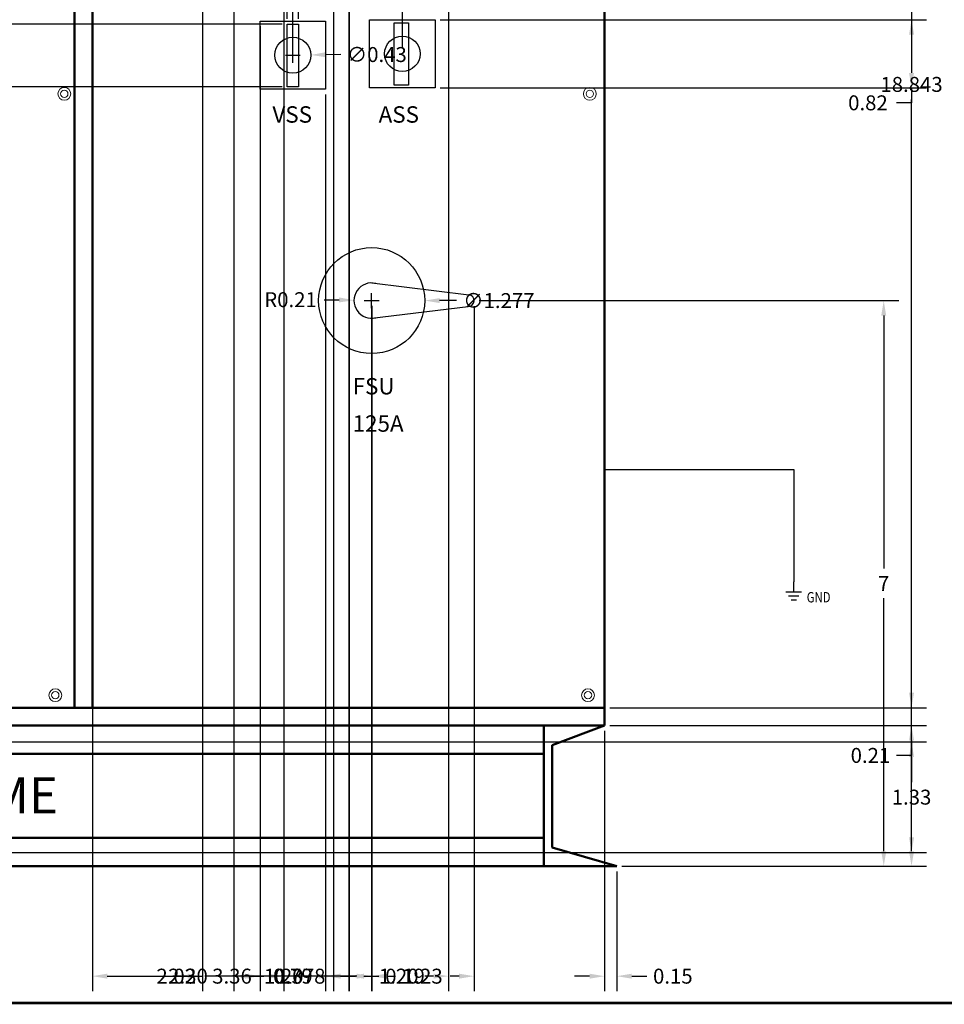
# Model space of a CAD drawing. Units: inches. Extents: x 0 to 33.5, y 0 to 22.4.
# Tile 4 of 6: x 16.8 to 27.9, y 0 to 11.9. Entities that reach past the tile are written whole.
import ezdxf
from ezdxf.enums import TextEntityAlignment as Align

# ---------------------------------------------------------------- set-up
doc = ezdxf.new("R2010")
doc.units = ezdxf.units.IN
doc.header["$MEASUREMENT"] = 0
for name, color, linetype, lineweight in [('E-ANNO-DIMS', 2, 'Continuous', 18), ('E-ANNO-TEXT', 7, 'Continuous', 18), ('E-ANNO-TTLB', 7, 'Continuous', 35), ('E-GRND-WIRE', 3, 'Continuous', 25), ('E-PANL-DEVC', 4, 'Continuous', 25), ('E-PANL-HDWR', 8, 'Continuous', 18), ('E-PANL-OUTL', 7, 'Continuous', 50), ('SYMS', 7, 'Continuous', 25)]:
    doc.layers.add(name, color=color, linetype=linetype, lineweight=lineweight)
doc.layers.add('TAGS', color=150, linetype='Continuous')
doc.layers.add('TITLE', color=7, linetype='Continuous')
doc.styles.add('ITALIC', font='ITALIC')
doc.styles.add('SIMPLEX', font='SIMPLEX')
doc.styles.add('WD', font='romans.shx')
doc.dimstyles.get("Standard").update_dxf_attribs({"dimtxt": 0.18, "dimasz": 0.18, "dimexe": 0.18, "dimexo": 0.0625, "dimgap": 0.09, "dimtad": 0, "dimtih": 1, "dimtoh": 1, "dimdec": 0, "dimzin": 0, "dimdsep": 46, "dimtxsty": 'Standard', "dimcen": 0.09, "dimadec": 0, "dimazin": 0, "dimtfac": 1, "dimtdec": 0, "dimtofl": 0, "dimtmove": 0, "dimatfit": 3, "dimfxl": 1, "dimtolj": 1, "dimtzin": 0, "dimarcsym": 0})

# ---------------------------------------------------------------- blocks, each defined once
blk = doc.blocks.new('NO_NUM_acade_title')
at = {"layer": 'TITLE', "const_width": 0.0312}
blk.add_lwpolyline([(30.594, 0.281), (30.594, 22.177), (30.344, 22.427), (0.281, 22.427), (0.031, 22.177), (0.031, 0.281), (0.281, 0.031), (30.344, 0.031)], close=True, dxfattribs=at)
at = {"layer": 'TITLE', "style": 'ITALIC'}
for tag, height, p in [('TITLE#1', 0.125, (32.156, 3.406)), ('TITLE#2', 0.125, (32.156, 3.204)), ('TITLE#3', 0.125, (32.156, 3.001)), ('TITLE#4', 0.125, (32.156, 2.799)), ('DWG#', 0.2, (32.156, 0.826))]:
    blk.add_attdef(tag, text='', height=height, dxfattribs=at).set_placement(p, align=Align.CENTER)
at = {"layer": 'TITLE', "style": 'SIMPLEX'}
blk.add_attdef('CAD#', (30.826, 1.958), '', height=0.0938, rotation=90, dxfattribs=at)
at = {"layer": 'TITLE'}
for tag, p, height, style in [('JOB#', (31.464, 1.644), 0.0938, 'SIMPLEX'), ('SCALE', (31.353, 1.344), 0.0938, 'SIMPLEX'), ('DATE', (32.408, 1.344), 0.0938, 'SIMPLEX'), ('SHTS', (32.532, 0.25), 0.2, 'ITALIC')]:
    blk.add_attdef(tag, p, '', height=height, dxfattribs=dict(at, style=style))
at = {"layer": 'TITLE', "style": 'ITALIC'}
blk.add_attdef('SH#', text='', height=0.2, dxfattribs=at).set_placement((31.881, 0.25), align=Align.RIGHT)
at = {"layer": 'TITLE', "flags": 9}
blk.add_attdef('WD_TB', (31.219, 0.031), '', height=0.125, dxfattribs=at)
blk = doc.blocks.new('VGND2')
for p, q in [((0, -0.125), (0, 0)), ((0.09375, -0.125), (-0.09375, -0.125)), ((-0.0625, -0.171875), (0.0625, -0.171875)), ((-0.03125, -0.21875), (0.03125, -0.21875))]:
    blk.add_line(p, q)
at = {"style": 'WD', "width": 0.8}
for tag, p in [('INST', (0.15625, 0.125)), ('LOC', (0.15625, -0.03125)), ('TAG1', (0.15625, -0.1875)), ('DESC1', (0.15625, -0.34375)), ('DESC2', (0.15625, -0.5))]:
    blk.add_attdef(tag, text='', height=0.125, dxfattribs=at).set_placement(p, align=Align.MIDDLE_LEFT)
at = {"style": 'WD', "flags": 1}
for tag in ['ASSYCODE', 'X2TERM01', 'CAT', 'MFG', 'FAMILY']:
    blk.add_attdef(tag, (0, 0), '', height=0.01, dxfattribs=at)
blk = doc.blocks.new('*D22')
at = {"layer": 'Defpoints', "color": 0, "transparency": 16777216}
for p in [(22.223, 8.496), (27.157, 8.496), (23.942, 1.68)]:
    blk.add_point(p, dxfattribs=at)
at = {"layer": 'E-ANNO-DIMS', "color": 0, "lineweight": -2, "transparency": 16777216}
for p, q in [((22.285, 8.496), (27.337, 8.496)), ((27.157, 8.316), (27.157, 5.268)), ((27.157, 1.86), (27.157, 4.908)), ((24.004, 1.68), (27.337, 1.68))]:
    blk.add_line(p, q, dxfattribs=at)
at = {"layer": 'E-ANNO-DIMS', "color": 0, "transparency": 16777216}
for points in [[(27.127, 8.316), (27.187, 8.316), (27.157, 8.496)], [(27.127, 1.86), (27.187, 1.86), (27.157, 1.68)]]:
    blk.add_solid(points, dxfattribs=at)
at = {"layer": 'E-ANNO-DIMS', "color": 0, "transparency": 16777216, "insert": (27.157, 5.088), "char_height": 0.18, "attachment_point": 5}
blk.add_mtext('\\A1;7', dxfattribs=at)
blk = doc.blocks.new('SCREW-PANEL')
for radius in [0.0768, 0.0442]:
    blk.add_circle((0.077, 0.077), radius)
blk = doc.blocks.new('*D31')
at = {"layer": 'Defpoints', "color": 0, "transparency": 16777216}
for p in [(14.887335, 20.522539), (27.49197, 20.522539), (23.941819, 1.679641)]:
    blk.add_point(p, dxfattribs=at)
at = {"layer": 'E-ANNO-DIMS', "color": 0, "lineweight": -2, "transparency": 16777216}
for p, q in [((14.949835, 20.522539), (27.67197, 20.522539)), ((27.49197, 20.342539), (27.49197, 11.28109)), ((27.49197, 1.859641), (27.49197, 10.92109)), ((24.004319, 1.679641), (27.67197, 1.679641))]:
    blk.add_line(p, q, dxfattribs=at)
at = {"layer": 'E-ANNO-DIMS', "color": 0, "transparency": 16777216}
for points in [[(27.46197, 20.342539), (27.52197, 20.342539), (27.49197, 20.522539)], [(27.46197, 1.859641), (27.52197, 1.859641), (27.49197, 1.679641)]]:
    blk.add_solid(points, dxfattribs=at)
at = {"layer": 'E-ANNO-DIMS', "color": 0, "transparency": 16777216, "insert": (27.49197, 11.10109), "char_height": 0.18, "attachment_point": 5}
blk.add_mtext('\\A1;18.843', dxfattribs=at)
blk = doc.blocks.new('*D32')
at = {"layer": 'Defpoints', "color": 0, "transparency": 16777216}
for p in [(23.793662, 3.589871), (23.793662, 3.375), (27.49197, 3.375)]:
    blk.add_point(p, dxfattribs=at)
at = {"layer": 'E-ANNO-DIMS', "color": 0, "lineweight": -2, "transparency": 16777216}
for p, q in [((27.49197, 3.769871), (27.49197, 3.949871)), ((23.856162, 3.589871), (27.67197, 3.589871)), ((23.856162, 3.375), (27.67197, 3.375)), ((27.49197, 3.195), (27.49197, 3.015)), ((27.49197, 3.015), (27.31197, 3.015))]:
    blk.add_line(p, q, dxfattribs=at)
at = {"layer": 'E-ANNO-DIMS', "color": 0, "transparency": 16777216}
for points in [[(27.46197, 3.769871), (27.52197, 3.769871), (27.49197, 3.589871)], [(27.46197, 3.195), (27.52197, 3.195), (27.49197, 3.375)]]:
    blk.add_solid(points, dxfattribs=at)
at = {"layer": 'E-ANNO-DIMS', "color": 0, "transparency": 16777216, "insert": (26.99697, 3.015), "char_height": 0.18, "attachment_point": 5}
blk.add_mtext('\\A1;0.21', dxfattribs=at)
blk = doc.blocks.new('*D33')
at = {"layer": 'Defpoints', "color": 0, "transparency": 16777216}
for p in [(23.061914, 3.375), (1.272879, 3.034671), (23.061914, 3.034671)]:
    blk.add_point(p, dxfattribs=at)
at = {"layer": 'E-ANNO-DIMS', "color": 0, "lineweight": -2, "transparency": 16777216}
for p, q in [((1.272879, 3.555), (1.272879, 3.735)), ((22.999414, 3.375), (1.092879, 3.375)), ((22.999414, 3.034671), (1.092879, 3.034671)), ((1.272879, 2.854671), (1.272879, 2.674671)), ((1.272879, 2.674671), (1.092879, 2.674671))]:
    blk.add_line(p, q, dxfattribs=at)
at = {"layer": 'E-ANNO-DIMS', "color": 0, "transparency": 16777216}
for points in [[(1.242879, 3.555), (1.302879, 3.555), (1.272879, 3.375)], [(1.242879, 2.854671), (1.302879, 2.854671), (1.272879, 3.034671)]]:
    blk.add_solid(points, dxfattribs=at)
at = {"layer": 'E-ANNO-DIMS', "color": 0, "transparency": 16777216, "insert": (0.747879, 2.674671), "char_height": 0.18, "attachment_point": 5}
blk.add_mtext('\\A1;0.34', dxfattribs=at)
blk = doc.blocks.new('*D34')
at = {"layer": 'Defpoints', "color": 0, "transparency": 16777216}
for p in [(23.061914, 2.019969), (1.272879, 1.679641), (23.061914, 1.679641)]:
    blk.add_point(p, dxfattribs=at)
at = {"layer": 'E-ANNO-DIMS', "color": 0, "lineweight": -2, "transparency": 16777216}
for p, q in [((1.272879, 2.199969), (1.272879, 2.379969)), ((22.999414, 2.019969), (1.092879, 2.019969)), ((22.999414, 1.679641), (1.092879, 1.679641)), ((1.272879, 1.499641), (1.272879, 1.319641)), ((1.272879, 1.319641), (1.092879, 1.319641))]:
    blk.add_line(p, q, dxfattribs=at)
at = {"layer": 'E-ANNO-DIMS', "color": 0, "transparency": 16777216}
for points in [[(1.242879, 2.199969), (1.302879, 2.199969), (1.272879, 2.019969)], [(1.242879, 1.499641), (1.302879, 1.499641), (1.272879, 1.679641)]]:
    blk.add_solid(points, dxfattribs=at)
at = {"layer": 'E-ANNO-DIMS', "color": 0, "transparency": 16777216, "insert": (0.747879, 1.319641), "char_height": 0.18, "attachment_point": 5}
blk.add_mtext('\\A1;0.34', dxfattribs=at)
blk = doc.blocks.new('*D37')
at = {"layer": 'Defpoints', "color": 0, "transparency": 16777216}
for p in [(5.494, 3.177), (5.494, 1.847), (27.492, 1.847)]:
    blk.add_point(p, dxfattribs=at)
at = {"layer": 'E-ANNO-DIMS', "color": 0, "lineweight": -2, "transparency": 16777216}
for p, q in [((5.557, 3.177), (27.672, 3.177)), ((27.492, 2.997), (27.492, 2.692)), ((27.492, 2.027), (27.492, 2.332)), ((5.557, 1.847), (27.672, 1.847))]:
    blk.add_line(p, q, dxfattribs=at)
at = {"layer": 'E-ANNO-DIMS', "color": 0, "transparency": 16777216}
for points in [[(27.462, 2.997), (27.522, 2.997), (27.492, 3.177)], [(27.462, 2.027), (27.522, 2.027), (27.492, 1.847)]]:
    blk.add_solid(points, dxfattribs=at)
at = {"layer": 'E-ANNO-DIMS', "color": 0, "transparency": 16777216, "insert": (27.492, 2.512), "char_height": 0.18, "attachment_point": 5}
blk.add_mtext('\\A1;1.33', dxfattribs=at)
blk = doc.blocks.new('*D38')
at = {"layer": 'Defpoints', "color": 0, "transparency": 16777216}
for p in [(23.793662, 3.375), (23.941819, 1.679641), (23.941819, 0.354641)]:
    blk.add_point(p, dxfattribs=at)
at = {"layer": 'E-ANNO-DIMS', "color": 0, "lineweight": -2, "transparency": 16777216}
for p, q in [((23.793662, 3.3125), (23.793662, 0.174641)), ((23.941819, 1.617141), (23.941819, 0.174641)), ((23.613662, 0.354641), (23.433662, 0.354641)), ((24.121819, 0.354641), (24.301819, 0.354641))]:
    blk.add_line(p, q, dxfattribs=at)
at = {"layer": 'E-ANNO-DIMS', "color": 0, "transparency": 16777216}
for points in [[(23.613662, 0.384641), (23.613662, 0.324641), (23.793662, 0.354641)], [(24.121819, 0.384641), (24.121819, 0.324641), (23.941819, 0.354641)]]:
    blk.add_solid(points, dxfattribs=at)
at = {"layer": 'E-ANNO-DIMS', "color": 0, "transparency": 16777216, "insert": (24.616819, 0.354641), "char_height": 0.18, "attachment_point": 5}
blk.add_mtext('\\A1;0.15', dxfattribs=at)
blk = doc.blocks.new('*D68')
at = {"layer": 'Defpoints', "color": 0, "transparency": 16777216}
for p in [(19.330943, 14.658017), (18.952991, 14.454443), (19.330943, 0.354641)]:
    blk.add_point(p, dxfattribs=at)
at = {"layer": 'E-ANNO-DIMS', "color": 0, "lineweight": -2, "transparency": 16777216}
for p, q in [((19.330943, 14.595517), (19.330943, 0.174641)), ((18.952991, 14.391943), (18.952991, 0.174641)), ((18.772991, 0.354641), (18.592991, 0.354641)), ((19.510943, 0.354641), (19.690943, 0.354641))]:
    blk.add_line(p, q, dxfattribs=at)
at = {"layer": 'E-ANNO-DIMS', "color": 0, "transparency": 16777216}
for points in [[(18.772991, 0.384641), (18.772991, 0.324641), (18.952991, 0.354641)], [(19.510943, 0.384641), (19.510943, 0.324641), (19.330943, 0.354641)]]:
    blk.add_solid(points, dxfattribs=at)
at = {"layer": 'E-ANNO-DIMS', "color": 0, "transparency": 16777216, "insert": (20.125943, 0.354641), "char_height": 0.18, "attachment_point": 5}
blk.add_mtext('\\A1;0.378', dxfattribs=at)
blk = doc.blocks.new('*D69')
at = {"layer": 'Defpoints', "color": 0, "transparency": 16777216}
for p in [(19.330943, 14.658017), (20.529167, 14.658017), (20.529167, 0.354641)]:
    blk.add_point(p, dxfattribs=at)
at = {"layer": 'E-ANNO-DIMS', "color": 0, "lineweight": -2, "transparency": 16777216}
for p, q in [((19.330943, 14.595517), (19.330943, 0.174641)), ((20.529167, 14.595517), (20.529167, 0.174641)), ((19.510943, 0.354641), (19.615055, 0.354641)), ((20.349167, 0.354641), (20.245055, 0.354641))]:
    blk.add_line(p, q, dxfattribs=at)
at = {"layer": 'E-ANNO-DIMS', "color": 0, "transparency": 16777216}
for points in [[(19.510943, 0.384641), (19.510943, 0.324641), (19.330943, 0.354641)], [(20.349167, 0.384641), (20.349167, 0.324641), (20.529167, 0.354641)]]:
    blk.add_solid(points, dxfattribs=at)
at = {"layer": 'E-ANNO-DIMS', "color": 0, "transparency": 16777216, "insert": (19.930055, 0.354641), "char_height": 0.18, "attachment_point": 5}
blk.add_mtext('\\A1;1.20', dxfattribs=at)
blk = doc.blocks.new('*D70')
at = {"layer": 'Defpoints', "color": 0, "transparency": 16777216}
for p in [(20.529167, 14.658017), (20.716317, 14.66483), (20.716317, 0.354641)]:
    blk.add_point(p, dxfattribs=at)
at = {"layer": 'E-ANNO-DIMS', "color": 0, "lineweight": -2, "transparency": 16777216}
for p, q in [((20.529167, 14.595517), (20.529167, 0.174641)), ((20.716317, 14.60233), (20.716317, 0.174641)), ((20.349167, 0.354641), (20.169167, 0.354641)), ((20.896317, 0.354641), (21.076317, 0.354641))]:
    blk.add_line(p, q, dxfattribs=at)
at = {"layer": 'E-ANNO-DIMS', "color": 0, "transparency": 16777216}
for points in [[(20.349167, 0.384641), (20.349167, 0.324641), (20.529167, 0.354641)], [(20.896317, 0.384641), (20.896317, 0.324641), (20.716317, 0.354641)]]:
    blk.add_solid(points, dxfattribs=at)
at = {"layer": 'E-ANNO-DIMS', "color": 0, "transparency": 16777216, "insert": (21.391317, 0.354641), "char_height": 0.18, "attachment_point": 5}
blk.add_mtext('\\A1;0.19', dxfattribs=at)
blk = doc.blocks.new('*D71')
at = {"layer": 'Defpoints', "color": 0, "transparency": 16777216}
for p in [(20.716, 14.665), (21.915, 14.665), (21.915, 0.355)]:
    blk.add_point(p, dxfattribs=at)
at = {"layer": 'E-ANNO-DIMS', "color": 0, "lineweight": -2, "transparency": 16777216}
for p, q in [((20.716, 14.602), (20.716, 0.175)), ((21.915, 14.602), (21.915, 0.175)), ((20.896, 0.355), (21, 0.355)), ((21.735, 0.355), (21.63, 0.355))]:
    blk.add_line(p, q, dxfattribs=at)
at = {"layer": 'E-ANNO-DIMS', "color": 0, "transparency": 16777216}
for points in [[(20.896, 0.385), (20.896, 0.325), (20.716, 0.355)], [(21.735, 0.385), (21.735, 0.325), (21.915, 0.355)]]:
    blk.add_solid(points, dxfattribs=at)
at = {"layer": 'E-ANNO-DIMS', "color": 0, "transparency": 16777216, "insert": (21.315, 0.355), "char_height": 0.18, "attachment_point": 5}
blk.add_mtext('\\A1;1.20', dxfattribs=at)
blk = doc.blocks.new('*D74')
at = {"layer": 'Defpoints', "color": 0, "transparency": 16777216}
for p in [(17.625, 18.375), (19.93, 13.017), (19.93, 0.355)]:
    blk.add_point(p, dxfattribs=at)
at = {"layer": 'E-ANNO-DIMS', "color": 0, "lineweight": -2, "transparency": 16777216}
for p, q in [((17.625, 18.312), (17.625, 0.175)), ((19.93, 12.954), (19.93, 0.175)), ((17.805, 0.355), (18.432, 0.355)), ((19.75, 0.355), (19.122, 0.355))]:
    blk.add_line(p, q, dxfattribs=at)
at = {"layer": 'E-ANNO-DIMS', "color": 0, "transparency": 16777216}
for points in [[(17.805, 0.385), (17.805, 0.325), (17.625, 0.355)], [(19.75, 0.385), (19.75, 0.325), (19.93, 0.355)]]:
    blk.add_solid(points, dxfattribs=at)
at = {"layer": 'E-ANNO-DIMS', "color": 0, "transparency": 16777216, "insert": (18.777, 0.355), "char_height": 0.18, "attachment_point": 5}
blk.add_mtext('\\A1;2.30', dxfattribs=at)
blk = doc.blocks.new('*D80')
at = {"layer": 'Defpoints', "color": 0, "transparency": 16777216}
for p in [(21.753278, 11.880921), (21.753278, 11.05915), (27.49197, 11.05915)]:
    blk.add_point(p, dxfattribs=at)
at = {"layer": 'E-ANNO-DIMS', "color": 0, "lineweight": -2, "transparency": 16777216}
for p, q in [((21.815778, 11.880921), (27.67197, 11.880921)), ((27.49197, 11.700921), (27.49197, 11.23915)), ((21.815778, 11.05915), (27.67197, 11.05915)), ((27.49197, 11.05915), (27.49197, 10.87915)), ((27.49197, 10.87915), (27.31197, 10.87915))]:
    blk.add_line(p, q, dxfattribs=at)
at = {"layer": 'E-ANNO-DIMS', "color": 0, "transparency": 16777216}
for points in [[(27.46197, 11.700921), (27.52197, 11.700921), (27.49197, 11.880921)], [(27.46197, 11.23915), (27.52197, 11.23915), (27.49197, 11.05915)]]:
    blk.add_solid(points, dxfattribs=at)
at = {"layer": 'E-ANNO-DIMS', "color": 0, "transparency": 16777216, "insert": (26.96697, 10.87915), "char_height": 0.18, "attachment_point": 5}
blk.add_mtext('\\A1;0.82', dxfattribs=at)
blk = doc.blocks.new('*D81')
at = {"layer": 'Defpoints', "color": 0, "transparency": 16777216}
for p in [(19.645, 11.042), (20.434, 11.042), (20.434, 0.355)]:
    blk.add_point(p, dxfattribs=at)
at = {"layer": 'E-ANNO-DIMS', "color": 0, "lineweight": -2, "transparency": 16777216}
for p, q in [((19.645, 10.98), (19.645, 0.175)), ((20.434, 10.98), (20.434, 0.175)), ((19.465, 0.355), (19.285, 0.355)), ((20.614, 0.355), (20.794, 0.355))]:
    blk.add_line(p, q, dxfattribs=at)
at = {"layer": 'E-ANNO-DIMS', "color": 0, "transparency": 16777216}
for points in [[(19.465, 0.385), (19.465, 0.325), (19.645, 0.355)], [(20.614, 0.385), (20.614, 0.325), (20.434, 0.355)]]:
    blk.add_solid(points, dxfattribs=at)
at = {"layer": 'E-ANNO-DIMS', "color": 0, "transparency": 16777216, "insert": (20.04, 0.355), "char_height": 0.18, "attachment_point": 5}
blk.add_mtext('\\A1;0.79', dxfattribs=at)
blk = doc.blocks.new('*D82')
at = {"layer": 'Defpoints', "color": 0, "transparency": 16777216}
for p in [(17.625, 18.375), (19.645494, 11.8638), (19.645494, 0.354641)]:
    blk.add_point(p, dxfattribs=at)
at = {"layer": 'E-ANNO-DIMS', "color": 0, "lineweight": -2, "transparency": 16777216}
for p, q in [((17.625, 18.3125), (17.625, 0.174641)), ((19.645494, 11.8013), (19.645494, 0.174641)), ((17.805, 0.354641), (18.290247, 0.354641)), ((19.465494, 0.354641), (18.980247, 0.354641))]:
    blk.add_line(p, q, dxfattribs=at)
at = {"layer": 'E-ANNO-DIMS', "color": 0, "transparency": 16777216}
for points in [[(17.805, 0.384641), (17.805, 0.324641), (17.625, 0.354641)], [(19.465494, 0.384641), (19.465494, 0.324641), (19.645494, 0.354641)]]:
    blk.add_solid(points, dxfattribs=at)
at = {"layer": 'E-ANNO-DIMS', "color": 0, "transparency": 16777216, "insert": (18.635247, 0.354641), "char_height": 0.18, "attachment_point": 5}
blk.add_mtext('\\A1;2.02', dxfattribs=at)
blk = doc.blocks.new('*D83')
at = {"layer": 'Defpoints', "color": 0, "transparency": 16777216}
for p in [(17.625, 18.375), (20.989, 8.496), (20.989, 0.355)]:
    blk.add_point(p, dxfattribs=at)
at = {"layer": 'E-ANNO-DIMS', "color": 0, "lineweight": -2, "transparency": 16777216}
for p, q in [((17.625, 18.312), (17.625, 0.175)), ((20.989, 8.433), (20.989, 0.175)), ((17.805, 0.355), (18.947, 0.355)), ((20.809, 0.355), (19.667, 0.355))]:
    blk.add_line(p, q, dxfattribs=at)
at = {"layer": 'E-ANNO-DIMS', "color": 0, "transparency": 16777216}
for points in [[(17.805, 0.385), (17.805, 0.325), (17.625, 0.355)], [(20.809, 0.385), (20.809, 0.325), (20.989, 0.355)]]:
    blk.add_solid(points, dxfattribs=at)
at = {"layer": 'E-ANNO-DIMS', "color": 0, "transparency": 16777216, "insert": (19.307, 0.355), "char_height": 0.18, "attachment_point": 5}
blk.add_mtext('\\A1;3.36', dxfattribs=at)
blk = doc.blocks.new('*D84')
at = {"layer": 'Defpoints', "color": 0, "transparency": 16777216}
for p in [(21.35914, 21.847539), (20.039632, 11.452915), (21.35914, 11.470035)]:
    blk.add_point(p, dxfattribs=at)
at = {"layer": 'E-ANNO-DIMS', "color": 0, "lineweight": -2, "transparency": 16777216}
for p, q in [((20.039632, 11.515415), (20.039632, 22.027539)), ((21.35914, 11.532535), (21.35914, 22.027539)), ((20.219632, 21.847539), (20.369386, 21.847539)), ((21.17914, 21.847539), (21.029386, 21.847539))]:
    blk.add_line(p, q, dxfattribs=at)
at = {"layer": 'E-ANNO-DIMS', "color": 0, "transparency": 16777216}
for points in [[(20.219632, 21.877539), (20.219632, 21.817539), (20.039632, 21.847539)], [(21.17914, 21.877539), (21.17914, 21.817539), (21.35914, 21.847539)]]:
    blk.add_solid(points, dxfattribs=at)
at = {"layer": 'E-ANNO-DIMS', "color": 0, "transparency": 16777216, "insert": (20.699386, 21.847539), "char_height": 0.18, "attachment_point": 5}
blk.add_mtext('\\A1;1.32', dxfattribs=at)
blk = doc.blocks.new('*D85')
at = {"layer": 'Defpoints', "color": 0, "transparency": 16777216}
for p in [(20.108027, 21.847539), (19.972101, 11.828212), (20.108027, 11.828212)]:
    blk.add_point(p, dxfattribs=at)
at = {"layer": 'E-ANNO-DIMS', "color": 0, "lineweight": -2, "transparency": 16777216}
for p, q in [((19.972101, 11.890712), (19.972101, 22.027539)), ((20.108027, 11.890712), (20.108027, 22.027539)), ((19.792101, 21.847539), (19.612101, 21.847539)), ((20.288027, 21.847539), (20.468027, 21.847539))]:
    blk.add_line(p, q, dxfattribs=at)
at = {"layer": 'E-ANNO-DIMS', "color": 0, "transparency": 16777216}
for points in [[(19.792101, 21.877539), (19.792101, 21.817539), (19.972101, 21.847539)], [(20.288027, 21.877539), (20.288027, 21.817539), (20.108027, 21.847539)]]:
    blk.add_solid(points, dxfattribs=at)
at = {"layer": 'E-ANNO-DIMS', "color": 0, "transparency": 16777216, "insert": (20.873027, 21.847539), "char_height": 0.18, "attachment_point": 5}
blk.add_mtext('\\A1;0.136', dxfattribs=at)
blk = doc.blocks.new('*D86')
at = {"layer": 'Defpoints', "color": 0, "transparency": 16777216}
for p in [(19.972101, 11.828212), (1.272879, 11.072826), (19.972101, 11.072826)]:
    blk.add_point(p, dxfattribs=at)
at = {"layer": 'E-ANNO-DIMS', "color": 0, "lineweight": -2, "transparency": 16777216}
for p, q in [((19.909601, 11.828212), (1.092879, 11.828212)), ((1.272879, 11.648212), (1.272879, 11.252826)), ((19.909601, 11.072826), (1.092879, 11.072826)), ((1.272879, 11.072826), (1.272879, 10.892826)), ((1.272879, 10.892826), (1.092879, 10.892826))]:
    blk.add_line(p, q, dxfattribs=at)
at = {"layer": 'E-ANNO-DIMS', "color": 0, "transparency": 16777216}
for points in [[(1.242879, 11.648212), (1.302879, 11.648212), (1.272879, 11.828212)], [(1.242879, 11.252826), (1.302879, 11.252826), (1.272879, 11.072826)]]:
    blk.add_solid(points, dxfattribs=at)
at = {"layer": 'E-ANNO-DIMS', "color": 0, "transparency": 16777216, "insert": (0.747879, 10.892826), "char_height": 0.18, "attachment_point": 5}
blk.add_mtext('\\A1;0.76', dxfattribs=at)
blk = doc.blocks.new('*D87')
at = {"layer": 'Defpoints', "color": 0, "transparency": 16777216}
for p in [(20.989405, 8.495777), (22.222557, 8.4915), (22.222557, 0.354641)]:
    blk.add_point(p, dxfattribs=at)
at = {"layer": 'E-ANNO-DIMS', "color": 0, "lineweight": -2, "transparency": 16777216}
for p, q in [((20.989405, 8.433277), (20.989405, 0.174641)), ((22.222557, 8.429), (22.222557, 0.174641)), ((21.169405, 0.354641), (21.275981, 0.354641)), ((22.042557, 0.354641), (21.935981, 0.354641))]:
    blk.add_line(p, q, dxfattribs=at)
at = {"layer": 'E-ANNO-DIMS', "color": 0, "transparency": 16777216}
for points in [[(21.169405, 0.384641), (21.169405, 0.324641), (20.989405, 0.354641)], [(22.042557, 0.384641), (22.042557, 0.324641), (22.222557, 0.354641)]]:
    blk.add_solid(points, dxfattribs=at)
at = {"layer": 'E-ANNO-DIMS', "color": 0, "transparency": 16777216, "insert": (21.605981, 0.354641), "char_height": 0.18, "attachment_point": 5}
blk.add_mtext('\\A1;1.23', dxfattribs=at)
blk = doc.blocks.new('*D98')
at = {"layer": 'Defpoints', "color": 0, "transparency": 16777216}
for p in [(19.823, 11.45), (20.256, 11.456)]:
    blk.add_point(p, dxfattribs=at)
at = {"layer": 'E-ANNO-DIMS', "color": 0, "lineweight": -2, "transparency": 16777216}
for p, q in [((20.04, 11.363), (20.04, 11.543)), ((19.95, 11.453), (20.13, 11.453)), ((20.616, 11.461), (20.436, 11.459))]:
    blk.add_line(p, q, dxfattribs=at)
at = {"layer": 'E-ANNO-DIMS', "color": 0, "transparency": 16777216}
blk.add_solid([(20.435, 11.489), (20.436, 11.429), (20.256, 11.456)], dxfattribs=at)
at = {"layer": 'E-ANNO-DIMS', "color": 0, "transparency": 16777216, "insert": (21.051, 11.461), "char_height": 0.18, "attachment_point": 5}
blk.add_mtext('\\A1;∅0.43', dxfattribs=at)
blk = doc.blocks.new('*D99')
at = {"layer": 'Defpoints', "color": 0, "transparency": 16777216}
for p in [(20.351, 8.496), (21.628, 8.496)]:
    blk.add_point(p, dxfattribs=at)
at = {"layer": 'E-ANNO-DIMS', "color": 0, "lineweight": -2, "transparency": 16777216}
for p, q in [((20.989, 8.406), (20.989, 8.586)), ((20.899, 8.496), (21.079, 8.496)), ((22.011, 8.496), (21.808, 8.496))]:
    blk.add_line(p, q, dxfattribs=at)
at = {"layer": 'E-ANNO-DIMS', "color": 0, "transparency": 16777216}
blk.add_solid([(21.808, 8.526), (21.808, 8.466), (21.628, 8.496)], dxfattribs=at)
at = {"layer": 'E-ANNO-DIMS', "color": 0, "transparency": 16777216, "insert": (22.521, 8.496), "char_height": 0.18, "attachment_point": 5}
blk.add_mtext('\\A1;∅1.277', dxfattribs=at)
blk = doc.blocks.new('*D100')
at = {"layer": 'Defpoints', "color": 0, "transparency": 16777216}
for p in [(20.777, 8.5), (20.989, 8.496)]:
    blk.add_point(p, dxfattribs=at)
at = {"layer": 'E-ANNO-DIMS', "color": 0, "lineweight": -2, "transparency": 16777216}
for p, q in [((20.989, 8.406), (20.989, 8.586)), ((20.417, 8.507), (20.597, 8.504)), ((20.899, 8.496), (21.079, 8.496))]:
    blk.add_line(p, q, dxfattribs=at)
at = {"layer": 'E-ANNO-DIMS', "color": 0, "transparency": 16777216}
blk.add_solid([(20.597, 8.534), (20.596, 8.474), (20.777, 8.5)], dxfattribs=at)
at = {"layer": 'E-ANNO-DIMS', "color": 0, "transparency": 16777216, "insert": (20.012, 8.507), "char_height": 0.18, "attachment_point": 5}
blk.add_mtext('\\A1;R0.21', dxfattribs=at)

msp = doc.modelspace()

# ---------------------------------------------------------------- linework, layer by layer
at = {"layer": 'E-GRND-WIRE'}
for p, q in [((23.7937, 6.4624), (23.7937, 6.4624)), ((23.7937, 6.4624), (26.0732, 6.4624)), ((26.0732, 6.4624), (26.0732, 5.1087))]:
    msp.add_line(p, q, dxfattribs=at)
at = {"layer": 'E-PANL-DEVC'}
for p, q in [((20.9894, 8.7087), (22.1607, 8.5658)), ((20.9894, 8.2829), (22.1522, 8.4253))]:
    msp.add_line(p, q, dxfattribs=at)
for points in [[(20.965, 11.8809), (21.7533, 11.8809), (21.7533, 11.0591), (20.965, 11.0591)], [(19.6455, 11.8638), (20.4338, 11.8638), (20.4338, 11.042), (19.6455, 11.042)], [(19.9721, 11.8282), (20.108, 11.8282), (20.108, 11.0728), (19.9721, 11.0728)], [(21.2623, 11.8436), (21.4319, 11.8436), (21.4319, 11.0939), (21.2623, 11.0939)]]:
    msp.add_lwpolyline(points, close=True, dxfattribs=at)
for centre, radius in [((20.0396, 11.4529), 0.2163), ((21.3591, 11.47), 0.2136), ((20.9894, 8.4958), 0.6385)]:
    msp.add_circle(centre, radius, dxfattribs=at)
for centre, radius, start, end in [((20.9894, 8.4958), 0.2129, 76.08855, 283.96221), ((22.1522, 8.4958), 0.0705, 270, 83.04427)]:
    msp.add_arc(centre, radius, start, end, dxfattribs=at)
at = {"layer": 'E-PANL-OUTL'}
for p, q in [((17.4101, 3.5899), (17.4101, 18.375)), ((17.625, 3.5899), (17.625, 18.375)), ((23.7937, 3.375), (23.7937, 18.375)), ((23.7937, 3.5899), (4.6251, 3.5899)), ((23.7937, 3.375), (4.6251, 3.375)), ((23.0619, 3.375), (23.0619, 1.6796)), ((23.7937, 3.375), (23.1623, 3.1365)), ((23.1623, 3.1365), (23.1623, 1.9046)), ((23.0619, 3.0347), (5.5819, 3.0347)), ((23.0619, 2.02), (5.5819, 2.02)), ((23.1623, 1.9046), (23.9418, 1.6796)), ((23.0619, 1.6796), (5.5819, 1.6796)), ((23.9418, 1.6796), (23.0619, 1.6796))]:
    msp.add_line(p, q, dxfattribs=at)

# ---------------------------------------------------------------- block references
at = {"layer": 'E-ANNO-TTLB'}
msp.add_blockref('NO_NUM_acade_title', (0, 0), dxfattribs=at)
at = {"layer": 'E-PANL-HDWR'}
for p in [(17.2103, 10.9105), (23.5401, 10.9105), (17.102, 3.6637), (23.518, 3.6637)]:
    msp.add_blockref('SCREW-PANEL', p, dxfattribs=at)
at = {"layer": 'SYMS'}
ref = msp.add_blockref('VGND2', (26.0732, 5.1087), dxfattribs=at)
ref.add_attrib('TAG1', 'GND', dxfattribs={"layer": 'TAGS', "height": 0.125, "style": 'WD', "width": 0.8}).set_placement((26.2295, 4.9212), align=Align.MIDDLE_LEFT)

# ---------------------------------------------------------------- texts
at = {"layer": 'E-ANNO-TEXT'}
for s, height, p in [('VSS', 0.19791, (19.7939, 10.6397)), ('ASS', 0.19791, (21.0732, 10.6397)), ('FSU', 0.19791, (20.7603, 7.3647)), ('125A', 0.19791, (20.7603, 6.9155)), ('BOLTED CHANNEL FRAME', 0.435566, (10.0718, 2.316))]:
    msp.add_text(s, height=height, dxfattribs=at).set_placement(p)

# ---------------------------------------------------------------- dimensions: what is measured, and where the dimension line sits
at = {"layer": 'E-ANNO-DIMS'}
for base, p1, p2, override, picture, middle in [((20.108, 21.8475), (19.9721, 11.8282), (20.108, 11.8282), {"dimdec": 3, "dimlfac": 1, "dimrnd": 0, "dimzin": 0, "dimdsep": 46, "dimlunit": 2}, '*D85', (20.873, 21.8475)), ((21.3591, 21.8475), (20.0396, 11.4529), (21.3591, 11.47), {"dimdec": 2, "dimlfac": 1, "dimrnd": 0, "dimzin": 0, "dimdsep": 46, "dimlunit": 2}, '*D84', (20.6994, 21.8475)), ((19.9297, 0.3546), (17.625, 18.375), (19.9297, 13.0169), {"dimdec": 2, "dimlfac": 1, "dimrnd": 0, "dimzin": 0, "dimdsep": 46, "dimlunit": 2}, '*D74', (18.7773, 0.3546)), ((19.6455, 0.3546), (17.625, 18.375), (19.6455, 11.8638), {"dimdec": 2, "dimlfac": 1, "dimrnd": 0, "dimzin": 0, "dimdsep": 46, "dimlunit": 2}, '*D82', (18.6352, 0.3546)), ((20.9894, 0.3546), (17.625, 18.375), (20.9894, 8.4958), {"dimdec": 2, "dimlfac": 1, "dimrnd": 0, "dimzin": 0, "dimdsep": 46, "dimlunit": 2}, '*D83', (19.3072, 0.3546)), ((19.3309, 0.3546), (18.953, 14.4544), (19.3309, 14.658), {"dimdec": 3, "dimlfac": 1, "dimrnd": 0, "dimzin": 0, "dimdsep": 46, "dimlunit": 2}, '*D68', (20.1259, 0.3546)), ((20.5292, 0.3546), (19.3309, 14.658), (20.5292, 14.658), {"dimdec": 2, "dimlfac": 1, "dimrnd": 0, "dimzin": 0, "dimdsep": 46, "dimlunit": 2}, '*D69', (19.9301, 0.3546)), ((20.7163, 0.3546), (20.5292, 14.658), (20.7163, 14.6648), {"dimdec": 2, "dimlfac": 1, "dimrnd": 0, "dimzin": 0, "dimdsep": 46, "dimlunit": 2}, '*D70', (21.3913, 0.3546)), ((21.9145, 0.3546), (20.7163, 14.6648), (21.9145, 14.6648), {"dimdec": 2, "dimlfac": 1, "dimrnd": 0, "dimzin": 0, "dimdsep": 46, "dimlunit": 2}, '*D71', (21.3154, 0.3546)), ((20.4338, 0.3546), (19.6455, 11.042), (20.4338, 11.042), {"dimdec": 2, "dimlfac": 1, "dimrnd": 0, "dimzin": 0, "dimdsep": 46, "dimlunit": 2}, '*D81', (20.0396, 0.3546)), ((22.2226, 0.3546), (20.9894, 8.4958), (22.2226, 8.4915), {"dimdec": 2, "dimlfac": 1, "dimrnd": 0, "dimzin": 0, "dimdsep": 46, "dimlunit": 2}, '*D87', (21.606, 0.3546)), ((23.9418, 0.3546), (23.7937, 3.375), (23.9418, 1.6796), {"dimdec": 2, "dimlfac": 1, "dimrnd": 0, "dimzin": 0, "dimdsep": 46, "dimlunit": 2}, '*D38', (24.6168, 0.3546))]:
    dim = msp.add_linear_dim(base=base, p1=p1, p2=p2, dimstyle='Standard', override=override, dxfattribs=at)
    dim.commit()
    dim.dimension.update_dxf_attribs({"geometry": picture, "text_midpoint": middle})
for base, p1, p2, override, picture, middle in [((27.492, 20.5225), (23.9418, 1.6796), (14.8873, 20.5225), {"dimdec": 3, "dimlfac": 1, "dimrnd": 0, "dimzin": 0, "dimdsep": 46, "dimlunit": 2}, '*D31', (27.492, 11.1011)), ((27.492, 11.0591), (21.7533, 11.8809), (21.7533, 11.0591), {"dimdec": 2, "dimlfac": 1, "dimrnd": 0, "dimzin": 0, "dimdsep": 46, "dimlunit": 2}, '*D80', (26.967, 10.8791)), ((1.2729, 11.0728), (19.9721, 11.8282), (19.9721, 11.0728), {"dimdec": 2, "dimlfac": 1, "dimrnd": 0, "dimzin": 0, "dimdsep": 46, "dimlunit": 2}, '*D86', (0.7479, 10.8928)), ((27.1566, 8.4958), (23.9418, 1.6796), (22.2227, 8.4958), {"dimclrd": 0, "dimclre": 0, "dimclrt": 0}, '*D22', (27.1566, 5.0877)), ((27.492, 3.375), (23.7937, 3.5899), (23.7937, 3.375), {"dimdec": 2, "dimlfac": 1, "dimrnd": 0, "dimzin": 0, "dimdsep": 46, "dimlunit": 2}, '*D32', (26.997, 3.015)), ((1.2729, 3.0347), (23.0619, 3.375), (23.0619, 3.0347), {"dimdec": 2, "dimlfac": 1, "dimrnd": 0, "dimzin": 0, "dimdsep": 46, "dimlunit": 2}, '*D33', (0.7479, 2.6747)), ((27.492, 1.8466), (5.4943, 3.1774), (5.4943, 1.8466), {"dimdec": 2, "dimlfac": 1, "dimrnd": 0, "dimzin": 0, "dimdsep": 46, "dimlunit": 2}, '*D37', (27.492, 2.512)), ((1.2729, 1.6796), (23.0619, 2.02), (23.0619, 1.6796), {"dimdec": 2, "dimlfac": 1, "dimrnd": 0, "dimzin": 0, "dimdsep": 46, "dimlunit": 2}, '*D34', (0.7479, 1.3196))]:
    dim = msp.add_linear_dim(base=base, p1=p1, p2=p2, angle=90, dimstyle='Standard', override=override, dxfattribs=at)
    dim.commit()
    dim.dimension.update_dxf_attribs({"geometry": picture, "text_midpoint": middle})
dim = msp.add_diameter_dim_2p(p1=(19.8234, 11.4498), p2=(20.2559, 11.456), dimstyle='Standard', override={"dimdec": 2, "dimlfac": 1, "dimrnd": 0, "dimzin": 0, "dimdsep": 46, "dimlunit": 2}, dxfattribs=at)
dim.commit()
dim.dimension.update_dxf_attribs({"geometry": '*D98', "text_midpoint": (20.6158, 11.4612)})
dim = msp.add_radius_dim(center=(20.9894, 8.4958), mpoint=(20.7766, 8.5), dimstyle='Standard', override={"dimdec": 2, "dimlfac": 1, "dimrnd": 0, "dimzin": 0, "dimdsep": 46, "dimlunit": 2}, dxfattribs=at)
dim.commit()
dim.dimension.update_dxf_attribs({"geometry": '*D100', "text_midpoint": (20.0116, 8.5071)})
dim = msp.add_diameter_dim_2p(p1=(20.3509, 8.4956), p2=(21.628, 8.496), dimstyle='Standard', override={"dimdec": 3, "dimlfac": 1, "dimrnd": 0, "dimzin": 0, "dimdsep": 46, "dimlunit": 2}, dxfattribs=at)
dim.commit()
dim.dimension.update_dxf_attribs({"geometry": '*D99', "text_midpoint": (22.0111, 8.4961), "dimtype": 163})

doc.saveas('drawing.dxf')
